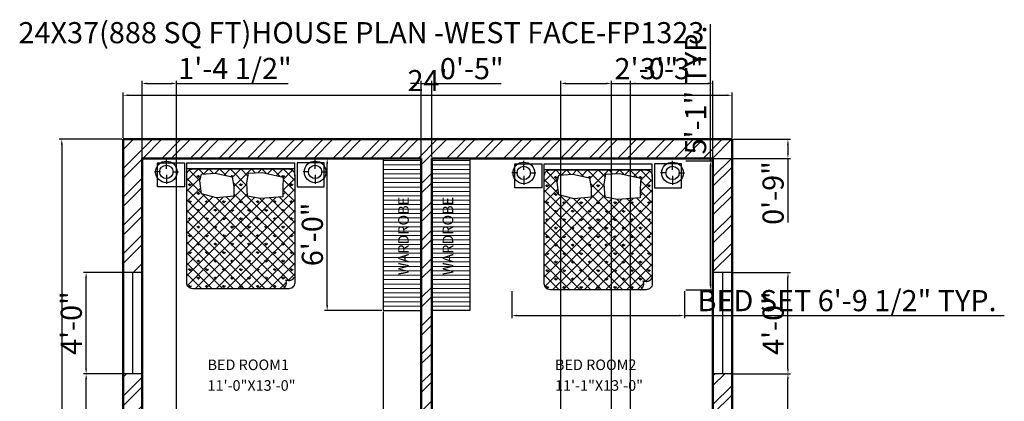
# Model space of a CAD drawing. Units: inches. Extents: x 3824 to 4289, y 1731 to 2259.
# Tile 5 of 5: x 3824 to 4289, y 2079 to 2259. Entities that reach past the tile are written whole.
import ezdxf

# ---------------------------------------------------------------- set-up
doc = ezdxf.new("R2010")
doc.units = ezdxf.units.IN
for name, color, linetype, lineweight in [('A-ANNO-DIMS', 2, 'Continuous', 18), ('A-ANNO-TEXT', 2, 'Continuous', 18), ('A-ANNO-TITL', 2, 'Continuous', 25), ('A-AREA-IDEN', 2, 'Continuous', 18), ('A-FLOR-CASE', 8, 'Continuous', 25), ('A-FURN', 9, 'Continuous', 18), ('WALL', 20, 'Continuous', 50), ('WINDOW', 4, 'Continuous', 25)]:
    doc.layers.add(name, color=color, linetype=linetype, lineweight=lineweight)
doc.layers.add('A-FLOR-CASE-PATT', color=251, linetype='Continuous', lineweight=13, true_color=0x636466)
doc.layers.add('A-WALL-PATT', color=251, linetype='Continuous', lineweight=13, true_color=0x636466)
doc.layers.add('GIUONG', color=70, linetype='Continuous')
doc.layers.add('NOI THAT', color=42, linetype='Continuous')
doc.styles.get("Standard").update_dxf_attribs({"font": 'arial.ttf'})
doc.dimstyles.new('ISO-25', dxfattribs={"dimtxt": 10, "dimasz": 2.5, "dimexe": 1.25, "dimexo": 0.625, "dimtad": 1, "dimdec": 1, "dimlunit": 3, "dimtxsty": 'Standard', "dimcen": 2.5, "dimadec": 0, "dimazin": 0, "dimtfac": 1, "dimtdec": 1, "dimtmove": 0, "dimatfit": 3, "dimfxl": 1, "dimarcsym": 0})

# ---------------------------------------------------------------- blocks, each defined once
blk = doc.blocks.new('*X4')
at = {"color": 0}
for p, q in [((0, 0), (0, 0)), ((-707, -141), (-734, -115)), ((-707, -141), (-707, -104)), ((-707, -141), (-681, -115)), ((-566, 0), (-566, 0)), ((-566, 0), (-566, 0)), ((-283, 0), (-283, 0)), ((-283, 0), (-283, 0)), ((-156, -126), (-168, -115)), ((-141, -141), (-142, -140)), ((-141, -141), (-141, -104)), ((-141, -141), (-115, -115)), ((120, -120), (115, -115)), ((283, 0), (283, 0)), ((566, 0), (566, 0)), ((699, -134), (681, -115)), ((707, -135), (707, -104)), ((710, -139), (734, -115)), ((-849, -283), (-875, -256)), ((-849, -283), (-849, -245)), ((-849, -283), (-822, -256)), ((0, -283), (-27, -256)), ((0, -283), (0, -245)), ((0, -283), (27, -256)), ((849, -283), (822, -256)), ((849, -283), (849, -245)), ((849, -283), (875, -256)), ((-707, -424), (-734, -398)), ((-707, -424), (-707, -387)), ((-707, -424), (-681, -398)), ((-116, -399), (-115, -398)), ((707, -424), (703, -420)), ((707, -424), (707, -387)), ((707, -424), (734, -398)), ((-849, -566), (-875, -539)), ((-849, -566), (-849, -528)), ((-849, -566), (-822, -539)), ((-566, -566), (-592, -539)), ((-566, -566), (-566, -528)), ((-566, -566), (-539, -539)), ((-283, -566), (-309, -539)), ((-283, -566), (-283, -528)), ((-283, -566), (-256, -539)), ((0, -566), (-27, -539)), ((0, -566), (0, -528)), ((0, -566), (27, -539)), ((283, -566), (256, -539)), ((283, -566), (283, -528)), ((283, -566), (309, -539)), ((566, -566), (539, -539)), ((566, -566), (566, -528)), ((566, -566), (592, -539)), ((849, -566), (822, -539)), ((849, -566), (849, -528)), ((849, -566), (875, -539)), ((-849, -849), (-849, -811)), ((-707, -707), (-734, -681)), ((-707, -707), (-707, -670)), ((-707, -707), (-681, -681)), ((-566, -849), (-566, -811)), ((-424, -707), (-451, -681)), ((-424, -707), (-424, -670)), ((-424, -707), (-398, -681)), ((-283, -849), (-283, -811)), ((-141, -707), (-168, -681)), ((-141, -707), (-141, -670)), ((-141, -707), (-115, -681)), ((0, -849), (0, -811)), ((141, -707), (115, -681)), ((141, -707), (141, -670)), ((141, -707), (168, -681)), ((283, -849), (283, -811)), ((424, -707), (398, -681)), ((424, -707), (424, -670)), ((424, -707), (451, -681)), ((566, -849), (566, -811)), ((707, -707), (681, -681)), ((707, -707), (707, -670)), ((707, -707), (734, -681)), ((849, -849), (849, -811)), ((-849, -849), (-875, -822)), ((-849, -849), (-822, -822)), ((-707, -990), (-734, -963)), ((-707, -990), (-707, -952)), ((-707, -990), (-681, -963)), ((-566, -849), (-592, -822)), ((-566, -849), (-539, -822)), ((-424, -990), (-451, -963)), ((-424, -990), (-424, -952)), ((-424, -990), (-398, -963)), ((-283, -849), (-309, -822)), ((-283, -849), (-256, -822)), ((-141, -990), (-168, -963)), ((-141, -990), (-141, -952)), ((-141, -990), (-115, -963)), ((0, -849), (-27, -822)), ((0, -849), (27, -822)), ((141, -990), (115, -963)), ((141, -990), (141, -952)), ((141, -990), (168, -963)), ((283, -849), (256, -822)), ((283, -849), (309, -822)), ((424, -990), (398, -963)), ((424, -990), (424, -952)), ((424, -990), (451, -963)), ((566, -849), (539, -822)), ((566, -849), (592, -822)), ((707, -990), (681, -963)), ((707, -990), (707, -952)), ((707, -990), (734, -963)), ((849, -849), (822, -822)), ((849, -849), (875, -822)), ((-849, -1131), (-875, -1105)), ((-849, -1131), (-849, -1094)), ((-849, -1131), (-822, -1105)), ((-566, -1131), (-592, -1105)), ((-566, -1131), (-566, -1094)), ((-566, -1131), (-539, -1105)), ((-283, -1131), (-309, -1105)), ((-283, -1131), (-283, -1094)), ((-283, -1131), (-256, -1105)), ((0, -1131), (-27, -1105)), ((0, -1131), (0, -1094)), ((0, -1131), (27, -1105)), ((283, -1131), (256, -1105)), ((283, -1131), (283, -1094)), ((283, -1131), (309, -1105)), ((566, -1131), (539, -1105)), ((566, -1131), (566, -1094)), ((566, -1131), (592, -1105)), ((849, -1131), (822, -1105)), ((849, -1131), (849, -1094)), ((849, -1131), (875, -1105)), ((-707, -1273), (-734, -1246)), ((-707, -1273), (-707, -1235)), ((-707, -1273), (-681, -1246)), ((-424, -1273), (-451, -1246)), ((-424, -1273), (-424, -1235)), ((-424, -1273), (-398, -1246)), ((-141, -1273), (-168, -1246)), ((-141, -1273), (-141, -1235)), ((-141, -1273), (-115, -1246)), ((141, -1273), (115, -1246)), ((141, -1273), (141, -1235)), ((141, -1273), (168, -1246)), ((424, -1273), (398, -1246)), ((424, -1273), (424, -1235)), ((424, -1273), (451, -1246)), ((707, -1273), (681, -1246)), ((707, -1273), (707, -1235)), ((707, -1273), (734, -1246)), ((-849, -1414), (-875, -1388)), ((-849, -1414), (-849, -1377)), ((-849, -1414), (-822, -1388)), ((-566, -1414), (-592, -1388)), ((-566, -1414), (-566, -1377)), ((-566, -1414), (-539, -1388)), ((-283, -1414), (-309, -1388)), ((-283, -1414), (-283, -1377)), ((-283, -1414), (-256, -1388)), ((0, -1414), (-27, -1388)), ((0, -1414), (0, -1377)), ((0, -1414), (27, -1388)), ((283, -1414), (256, -1388)), ((283, -1414), (283, -1377)), ((283, -1414), (309, -1388)), ((566, -1414), (539, -1388)), ((566, -1414), (566, -1377)), ((566, -1414), (592, -1388)), ((849, -1414), (822, -1388)), ((849, -1414), (849, -1377)), ((849, -1414), (875, -1388)), ((-707, -1556), (-734, -1529)), ((-707, -1556), (-707, -1518)), ((-707, -1556), (-681, -1529)), ((-424, -1556), (-451, -1529)), ((-424, -1556), (-424, -1518)), ((-424, -1556), (-398, -1529)), ((-141, -1556), (-168, -1529)), ((-141, -1556), (-141, -1518)), ((-141, -1556), (-115, -1529)), ((141, -1556), (115, -1529)), ((141, -1556), (141, -1518)), ((141, -1556), (168, -1529)), ((424, -1556), (398, -1529)), ((424, -1556), (424, -1518)), ((424, -1556), (451, -1529)), ((707, -1556), (681, -1529)), ((707, -1556), (707, -1518)), ((707, -1556), (734, -1529)), ((-849, -1697), (-875, -1671)), ((-849, -1697), (-849, -1660)), ((-849, -1697), (-822, -1671)), ((-707, -1838), (-707, -1801)), ((-566, -1697), (-592, -1671)), ((-566, -1697), (-566, -1660)), ((-566, -1697), (-539, -1671)), ((-424, -1838), (-424, -1801)), ((-283, -1697), (-309, -1671)), ((-283, -1697), (-283, -1660)), ((-283, -1697), (-256, -1671)), ((-141, -1838), (-141, -1801)), ((0, -1697), (-27, -1671)), ((0, -1697), (0, -1660)), ((0, -1697), (27, -1671)), ((141, -1838), (141, -1801)), ((283, -1697), (256, -1671)), ((283, -1697), (283, -1660)), ((283, -1697), (309, -1671)), ((424, -1838), (424, -1801)), ((566, -1697), (539, -1671)), ((566, -1697), (566, -1660)), ((566, -1697), (592, -1671)), ((707, -1838), (707, -1801)), ((849, -1697), (822, -1671)), ((849, -1697), (849, -1660)), ((849, -1697), (875, -1671)), ((-849, -1980), (-875, -1953)), ((-849, -1980), (-849, -1942)), ((-849, -1980), (-822, -1953)), ((-707, -1838), (-734, -1812)), ((-707, -1838), (-681, -1812)), ((-566, -1980), (-592, -1953)), ((-566, -1980), (-566, -1942)), ((-566, -1980), (-539, -1953)), ((-424, -1838), (-451, -1812)), ((-424, -1838), (-398, -1812)), ((-283, -1980), (-309, -1953)), ((-283, -1980), (-283, -1942)), ((-283, -1980), (-256, -1953)), ((-141, -1838), (-168, -1812)), ((-141, -1838), (-115, -1812)), ((0, -1980), (-27, -1953)), ((0, -1980), (0, -1942)), ((0, -1980), (27, -1953)), ((141, -1838), (115, -1812)), ((141, -1838), (168, -1812)), ((283, -1980), (256, -1953)), ((283, -1980), (283, -1942)), ((283, -1980), (309, -1953)), ((424, -1838), (398, -1812)), ((424, -1838), (451, -1812)), ((566, -1980), (539, -1953)), ((566, -1980), (566, -1942)), ((566, -1980), (592, -1953)), ((707, -1838), (681, -1812)), ((707, -1838), (734, -1812))]:
    blk.add_line(p, q, dxfattribs=at)
blk = doc.blocks.new('*X3')
at = {"color": 0}
for p, q in [((-900, -193), (-707, 0)), ((-623, -84), (-707, 0)), ((-614, -83), (-530, 0)), ((-457, -74), (-530, 0)), ((-425, -72), (-354, 0)), ((-245, -108), (-354, 0)), ((-278, -101), (-177, 0)), ((103, -280), (-177, 0)), ((-142, -142), (0, 0)), ((-117, -294), (177, 0)), ((120, -120), (0, 0)), ((241, -64), (177, 0)), ((292, -61), (354, 0)), ((426, -72), (354, 0)), ((452, -78), (530, 0)), ((654, -123), (530, 0)), ((596, -111), (707, 0)), ((900, -193), (707, 0)), ((-900, -370), (-667, -137)), ((-656, -405), (-900, -161)), ((-683, -201), (-862, -22)), ((703, -358), (900, -161)), ((708, -175), (862, -22)), ((-900, -1254), (101, -252)), ((-900, -546), (-668, -314)), ((900, -1254), (-128, -225)), ((900, -370), (708, -178)), ((735, -1973), (-900, -337)), ((-900, -1430), (112, -418)), ((-900, -723), (-605, -429)), ((-900, -900), (-465, -465)), ((-900, -1077), (-293, -470)), ((-900, -1607), (231, -476)), ((-900, -1784), (394, -489)), ((-888, -1948), (586, -475)), ((-763, -2000), (900, -337)), ((801, -1862), (-641, -419)), ((900, -1784), (-404, -480)), ((900, -1607), (-243, -465)), ((900, -1430), (-116, -415)), ((900, -900), (483, -483)), ((900, -723), (647, -470)), ((900, -546), (703, -349)), ((586, -2000), (-900, -514)), ((-586, -2000), (900, -514)), ((900, -1077), (317, -494)), ((409, -2000), (-900, -691)), ((-409, -2000), (900, -691)), ((232, -2000), (-900, -868)), ((-232, -2000), (900, -868)), ((55, -2000), (-900, -1045)), ((-55, -2000), (900, -1045)), ((-121, -2000), (-900, -1221)), ((121, -2000), (900, -1221)), ((-298, -2000), (-900, -1398)), ((298, -2000), (900, -1398)), ((-475, -2000), (-900, -1575)), ((475, -2000), (900, -1575)), ((-652, -2000), (-900, -1752)), ((790, -1861), (900, -1752)), ((-835, -1994), (-894, -1935)), ((652, -2000), (761, -1890))]:
    blk.add_line(p, q, dxfattribs=at)
blk = doc.blocks.new('A$C190D2546')
at = {"layer": 'GIUONG'}
for points in [[(787, 1584), (758, 1799), (787, 1914), (1016, 1928), (1296, 1871), (1325, 1699), (1325, 1548), (1038, 1519)], [(1555, 1548), (1541, 1771), (1569, 1928), (1799, 1943), (2151, 1864), (2144, 1685), (2144, 1534), (1763, 1505)]]:
    blk.add_lwpolyline(points, close=True, dxfattribs=at)
for centre, radius in [((200, 1951), 180), ((200, 1951), 112), ((2682, 1951), 180), ((2682, 1951), 112)]:
    blk.add_circle(centre, radius, dxfattribs=at)
at = {"layer": 'NOI THAT'}
for p, q in [((200, 2001), (200, 2151)), ((2682, 2001), (2682, 2151)), ((541, 2100), (2341, 2100)), ((541, 1881), (541, 2100)), ((2341, 2000), (541, 2000)), ((2341, 1881), (2341, 2100)), ((100, 1951), (0, 1951)), ((200, 1901), (200, 1751)), ((300, 1951), (400, 1951)), ((2582, 1951), (2482, 1951)), ((2682, 1901), (2682, 1751)), ((2782, 1951), (2882, 1951))]:
    blk.add_line(p, q, dxfattribs=at)
for points in [[(500, 2101), (500, 1701), (50, 1701), (50, 2101)], [(2382, 2101), (2382, 1701), (2832, 1701), (2832, 2101)]]:
    blk.add_lwpolyline(points, close=True, dxfattribs=at)
blk.add_lwpolyline([(641, 2000), (2241, 2000, -0.414214), (2341, 1900), (2341, 100, -0.414214), (2241, 0), (641, 0, -0.414214), (541, 100), (541, 1900, -0.414214)], format="xyb", close=True, dxfattribs=at)
for centre, start, end in [((2241, 250), 243.4349, 333.4349), ((2091, 100), 296.5651, 26.5651)]:
    blk.add_arc(centre, 112, start, end, dxfattribs=at)
for name in ['*X3', '*X4']:
    blk.add_blockref(name, (1441, 2000), dxfattribs=at)
blk = doc.blocks.new('*D11')
at = {"layer": 'A-ANNO-DIMS', "color": 0, "lineweight": -2, "transparency": 16777216}
for p, q in [((3872.55, 2203.24), (3872.55, 2224.73)), ((3875.05, 2223.48), (4158.05, 2223.48)), ((4160.55, 2203.24), (4160.55, 2224.73))]:
    blk.add_line(p, q, dxfattribs=at)
at = {"layer": 'A-ANNO-DIMS', "color": 0, "transparency": 16777216}
for points in [[(3875.05, 2223.9), (3875.05, 2223.07), (3872.55, 2223.48)], [(4158.05, 2223.9), (4158.05, 2223.07), (4160.55, 2223.48)]]:
    blk.add_solid(points, dxfattribs=at)
at = {"layer": 'Defpoints', "color": 0, "transparency": 16777216}
for p in [(4160.55, 2223.48), (3872.55, 2202.62), (4160.55, 2202.62)]:
    blk.add_point(p, dxfattribs=at)
at = {"layer": 'A-ANNO-DIMS', "color": 0, "transparency": 16777216, "insert": (4016.55, 2229.13), "char_height": 10, "attachment_point": 5}
blk.add_mtext("24'", dxfattribs=at)
blk = doc.blocks.new('*D12')
at = {"layer": 'A-ANNO-DIMS', "color": 0, "lineweight": -2, "transparency": 16777216}
for p, q in [((3871.93, 2202.62), (3842.32, 2202.62)), ((3843.57, 2200.12), (3843.57, 1761.12)), ((3871.93, 1758.62), (3842.32, 1758.62))]:
    blk.add_line(p, q, dxfattribs=at)
at = {"layer": 'A-ANNO-DIMS', "color": 0, "transparency": 16777216}
for points in [[(3843.15, 2200.12), (3843.99, 2200.12), (3843.57, 2202.62)], [(3843.15, 1761.12), (3843.99, 1761.12), (3843.57, 1758.62)]]:
    blk.add_solid(points, dxfattribs=at)
at = {"layer": 'Defpoints', "color": 0, "transparency": 16777216}
for p in [(3872.55, 2202.62), (3843.57, 1758.62), (3872.55, 1758.62)]:
    blk.add_point(p, dxfattribs=at)
at = {"layer": 'A-ANNO-DIMS', "color": 0, "transparency": 16777216, "insert": (3837.84, 1980.62), "char_height": 10, "attachment_point": 5, "rotation": 90}
blk.add_mtext("37'", dxfattribs=at)
blk = doc.blocks.new('*D14')
at = {"layer": 'A-ANNO-DIMS', "color": 0, "lineweight": -2, "transparency": 16777216}
for p, q in [((4056.41, 2130.79), (4056.41, 2117.92)), ((4138.1, 2130.79), (4138.1, 2117.92)), ((4058.91, 2119.17), (4135.6, 2119.17)), ((4138.1, 2119.17), (4289.32, 2119.17))]:
    blk.add_line(p, q, dxfattribs=at)
at = {"layer": 'A-ANNO-DIMS', "color": 0, "transparency": 16777216}
for points in [[(4058.91, 2119.58), (4058.91, 2118.75), (4056.41, 2119.17)], [(4135.6, 2119.58), (4135.6, 2118.75), (4138.1, 2119.17)]]:
    blk.add_solid(points, dxfattribs=at)
at = {"layer": 'Defpoints', "color": 0, "transparency": 16777216}
for p in [(4056.41, 2131.42), (4138.1, 2131.42), (4138.1, 2119.17)]:
    blk.add_point(p, dxfattribs=at)
at = {"layer": 'A-ANNO-DIMS', "color": 0, "transparency": 16777216, "insert": (4214.96, 2124.96), "char_height": 10, "attachment_point": 5}
blk.add_mtext('BED SET 6\'-9 1/2" TYP.', dxfattribs=at)
blk = doc.blocks.new('*D15')
at = {"layer": 'A-ANNO-DIMS', "color": 0, "lineweight": -2, "transparency": 16777216}
for p, q in [((4150.35, 2192.38), (4150.35, 2257.09)), ((4138.72, 2192.38), (4151.6, 2192.38)), ((4150.35, 2133.92), (4150.35, 2189.88)), ((4138.72, 2131.42), (4151.6, 2131.42))]:
    blk.add_line(p, q, dxfattribs=at)
at = {"layer": 'A-ANNO-DIMS', "color": 0, "transparency": 16777216}
for points in [[(4149.93, 2189.88), (4150.77, 2189.88), (4150.35, 2192.38)], [(4149.93, 2133.92), (4150.77, 2133.92), (4150.35, 2131.42)]]:
    blk.add_solid(points, dxfattribs=at)
at = {"layer": 'Defpoints', "color": 0, "transparency": 16777216}
for p in [(4138.1, 2192.38), (4150.35, 2192.38), (4138.1, 2131.42)]:
    blk.add_point(p, dxfattribs=at)
at = {"layer": 'A-ANNO-DIMS', "color": 0, "transparency": 16777216, "insert": (4144.62, 2225.98), "char_height": 10, "attachment_point": 5, "rotation": 90}
blk.add_mtext('5\'-1" TYP.', dxfattribs=at)
blk = doc.blocks.new('*D30')
at = {"layer": 'A-ANNO-DIMS', "color": 0, "lineweight": -2, "transparency": 16777216}
for p, q in [((3880.93, 2091.62), (3853.85, 2091.62)), ((3855.1, 2017.12), (3855.1, 2089.12)), ((3880.93, 2014.62), (3853.85, 2014.62))]:
    blk.add_line(p, q, dxfattribs=at)
at = {"layer": 'A-ANNO-DIMS', "color": 0, "transparency": 16777216}
for points in [[(3854.69, 2089.12), (3855.52, 2089.12), (3855.1, 2091.62)], [(3854.69, 2017.12), (3855.52, 2017.12), (3855.1, 2014.62)]]:
    blk.add_solid(points, dxfattribs=at)
at = {"layer": 'Defpoints', "color": 0, "transparency": 16777216}
for p in [(3855.1, 2091.62), (3881.55, 2091.62), (3881.55, 2014.62)]:
    blk.add_point(p, dxfattribs=at)
at = {"layer": 'A-ANNO-DIMS', "color": 0, "transparency": 16777216, "insert": (3849.37, 2053.12), "char_height": 10, "attachment_point": 5, "rotation": 90}
blk.add_mtext('6\'-5"', dxfattribs=at)
blk = doc.blocks.new('*D31')
at = {"layer": 'A-ANNO-DIMS', "color": 0, "lineweight": -2, "transparency": 16777216}
for p, q in [((3880.93, 2139.62), (3853.85, 2139.62)), ((3855.1, 2094.12), (3855.1, 2137.12)), ((3880.93, 2091.62), (3853.85, 2091.62))]:
    blk.add_line(p, q, dxfattribs=at)
at = {"layer": 'A-ANNO-DIMS', "color": 0, "transparency": 16777216}
for points in [[(3854.69, 2137.12), (3855.52, 2137.12), (3855.1, 2139.62)], [(3854.69, 2094.12), (3855.52, 2094.12), (3855.1, 2091.62)]]:
    blk.add_solid(points, dxfattribs=at)
at = {"layer": 'Defpoints', "color": 0, "transparency": 16777216}
for p in [(3855.1, 2139.62), (3881.55, 2139.62), (3881.55, 2091.62)]:
    blk.add_point(p, dxfattribs=at)
at = {"layer": 'A-ANNO-DIMS', "color": 0, "transparency": 16777216, "insert": (3849.37, 2115.62), "char_height": 10, "attachment_point": 5, "rotation": 90}
blk.add_mtext('4\'-0"', dxfattribs=at)
blk = doc.blocks.new('*D36')
at = {"layer": 'A-ANNO-DIMS', "color": 0, "lineweight": -2, "transparency": 16777216}
for p, q in [((4161.18, 2091.62), (4188.25, 2091.62)), ((4187, 2011.12), (4187, 2089.12)), ((4161.18, 2008.62), (4188.25, 2008.62))]:
    blk.add_line(p, q, dxfattribs=at)
at = {"layer": 'A-ANNO-DIMS', "color": 0, "transparency": 16777216}
for points in [[(4186.59, 2089.12), (4187.42, 2089.12), (4187, 2091.62)], [(4186.59, 2011.12), (4187.42, 2011.12), (4187, 2008.62)]]:
    blk.add_solid(points, dxfattribs=at)
at = {"layer": 'Defpoints', "color": 0, "transparency": 16777216}
for p in [(4160.55, 2091.62), (4187, 2091.62), (4160.55, 2008.62)]:
    blk.add_point(p, dxfattribs=at)
at = {"layer": 'A-ANNO-DIMS', "color": 0, "transparency": 16777216, "insert": (4181.27, 2050.12), "char_height": 10, "attachment_point": 5, "rotation": 90}
blk.add_mtext('6\'-11"', dxfattribs=at)
blk = doc.blocks.new('*D37')
at = {"layer": 'A-ANNO-DIMS', "color": 0, "lineweight": -2, "transparency": 16777216}
for p, q in [((4161.18, 2139.62), (4188.25, 2139.62)), ((4187, 2094.12), (4187, 2137.12)), ((4161.18, 2091.62), (4188.25, 2091.62))]:
    blk.add_line(p, q, dxfattribs=at)
at = {"layer": 'A-ANNO-DIMS', "color": 0, "transparency": 16777216}
for points in [[(4186.59, 2137.12), (4187.42, 2137.12), (4187, 2139.62)], [(4186.59, 2094.12), (4187.42, 2094.12), (4187, 2091.62)]]:
    blk.add_solid(points, dxfattribs=at)
at = {"layer": 'Defpoints', "color": 0, "transparency": 16777216}
for p in [(4160.55, 2139.62), (4187, 2139.62), (4160.55, 2091.62)]:
    blk.add_point(p, dxfattribs=at)
at = {"layer": 'A-ANNO-DIMS', "color": 0, "transparency": 16777216, "insert": (4181.27, 2115.62), "char_height": 10, "attachment_point": 5, "rotation": 90}
blk.add_mtext('4\'-0"', dxfattribs=at)
blk = doc.blocks.new('*D50')
at = {"layer": 'A-ANNO-DIMS', "color": 0, "lineweight": -2, "transparency": 16777216}
for p, q in [((4079.55, 1818.24), (4079.55, 2230.32)), ((4082.05, 2229.07), (4101.05, 2229.07)), ((4103.55, 1818.24), (4103.55, 2230.32)), ((4103.55, 2229.07), (4134.06, 2229.07))]:
    blk.add_line(p, q, dxfattribs=at)
at = {"layer": 'A-ANNO-DIMS', "color": 0, "transparency": 16777216}
for points in [[(4082.05, 2229.49), (4082.05, 2228.65), (4079.55, 2229.07)], [(4101.05, 2229.49), (4101.05, 2228.65), (4103.55, 2229.07)]]:
    blk.add_solid(points, dxfattribs=at)
at = {"layer": 'Defpoints', "color": 0, "transparency": 16777216}
for p in [(4103.55, 2229.07), (4079.55, 1817.62), (4103.55, 1817.62)]:
    blk.add_point(p, dxfattribs=at)
at = {"layer": 'A-ANNO-DIMS', "color": 0, "transparency": 16777216, "insert": (4120.05, 2234.8), "char_height": 10, "attachment_point": 5}
blk.add_mtext('2\'-0"', dxfattribs=at)
blk = doc.blocks.new('*D51')
at = {"layer": 'A-ANNO-DIMS', "color": 0, "lineweight": -2, "transparency": 16777216}
for p, q in [((4112.55, 1917.24), (4112.55, 2230.32)), ((4115.05, 2229.07), (4149.05, 2229.07)), ((4151.55, 1917.24), (4151.55, 2230.32))]:
    blk.add_line(p, q, dxfattribs=at)
at = {"layer": 'A-ANNO-DIMS', "color": 0, "transparency": 16777216}
for points in [[(4115.05, 2229.49), (4115.05, 2228.65), (4112.55, 2229.07)], [(4149.05, 2229.49), (4149.05, 2228.65), (4151.55, 2229.07)]]:
    blk.add_solid(points, dxfattribs=at)
at = {"layer": 'Defpoints', "color": 0, "transparency": 16777216}
for p in [(4151.55, 2229.07), (4112.55, 1916.62), (4151.55, 1916.62)]:
    blk.add_point(p, dxfattribs=at)
at = {"layer": 'A-ANNO-DIMS', "color": 0, "transparency": 16777216, "insert": (4132.05, 2234.8), "char_height": 10, "attachment_point": 5}
blk.add_mtext('3\'-3"', dxfattribs=at)
blk = doc.blocks.new('*D54')
at = {"layer": 'A-ANNO-DIMS', "color": 0, "lineweight": -2, "transparency": 16777216}
for p, q in [((4161.18, 2202.62), (4188.25, 2202.62)), ((4187, 2200.12), (4187, 2196.12)), ((4152.18, 2193.62), (4188.25, 2193.62)), ((4187, 2193.62), (4187, 2163.29))]:
    blk.add_line(p, q, dxfattribs=at)
at = {"layer": 'A-ANNO-DIMS', "color": 0, "transparency": 16777216}
for points in [[(4186.59, 2200.12), (4187.42, 2200.12), (4187, 2202.62)], [(4186.59, 2196.12), (4187.42, 2196.12), (4187, 2193.62)]]:
    blk.add_solid(points, dxfattribs=at)
at = {"layer": 'Defpoints', "color": 0, "transparency": 16777216}
for p in [(4160.55, 2202.62), (4151.55, 2193.62), (4187, 2193.62)]:
    blk.add_point(p, dxfattribs=at)
at = {"layer": 'A-ANNO-DIMS', "color": 0, "transparency": 16777216, "insert": (4181.27, 2177.2), "char_height": 10, "attachment_point": 5, "rotation": 90}
blk.add_mtext('0\'-9"', dxfattribs=at)
blk = doc.blocks.new('*D55')
at = {"layer": 'A-ANNO-DIMS', "color": 0, "lineweight": -2, "transparency": 16777216}
for p, q in [((4011.05, 2229.07), (4008.55, 2229.07)), ((4013.55, 2194.24), (4013.55, 2230.32)), ((4013.55, 2229.07), (4018.55, 2229.07)), ((4018.55, 2194.24), (4018.55, 2230.32)), ((4021.05, 2229.07), (4051.38, 2229.07))]:
    blk.add_line(p, q, dxfattribs=at)
at = {"layer": 'A-ANNO-DIMS', "color": 0, "transparency": 16777216}
for points in [[(4011.05, 2229.49), (4011.05, 2228.65), (4013.55, 2229.07)], [(4021.05, 2229.49), (4021.05, 2228.65), (4018.55, 2229.07)]]:
    blk.add_solid(points, dxfattribs=at)
at = {"layer": 'Defpoints', "color": 0, "transparency": 16777216}
for p in [(4018.55, 2229.07), (4013.55, 2193.62), (4018.55, 2193.62)]:
    blk.add_point(p, dxfattribs=at)
at = {"layer": 'A-ANNO-DIMS', "color": 0, "transparency": 16777216, "insert": (4037.47, 2234.8), "char_height": 10, "attachment_point": 5}
blk.add_mtext('0\'-5"', dxfattribs=at)
blk = doc.blocks.new('*D56')
at = {"layer": 'A-ANNO-DIMS', "color": 0, "lineweight": -2, "transparency": 16777216}
for p, q in [((3995.55, 2120.99), (3995.55, 1730.92)), ((4013.55, 2120.99), (4013.55, 1730.92)), ((3998.05, 1732.17), (4011.05, 1732.17)), ((4013.55, 1732.17), (4042.94, 1732.17))]:
    blk.add_line(p, q, dxfattribs=at)
at = {"layer": 'A-ANNO-DIMS', "color": 0, "transparency": 16777216}
for points in [[(3998.05, 1732.59), (3998.05, 1731.75), (3995.55, 1732.17)], [(4011.05, 1732.59), (4011.05, 1731.75), (4013.55, 1732.17)]]:
    blk.add_solid(points, dxfattribs=at)
at = {"layer": 'Defpoints', "color": 0, "transparency": 16777216}
for p in [(3995.55, 2121.62), (4013.55, 2121.62), (4013.55, 1732.17)]:
    blk.add_point(p, dxfattribs=at)
at = {"layer": 'A-ANNO-DIMS', "color": 0, "transparency": 16777216, "insert": (4029.5, 1737.9), "char_height": 10, "attachment_point": 5}
blk.add_mtext('1\'-6"', dxfattribs=at)
blk = doc.blocks.new('*D57')
at = {"layer": 'A-ANNO-DIMS', "color": 0, "lineweight": -2, "transparency": 16777216}
for p, q in [((3994.93, 2193.62), (3967.85, 2193.62)), ((3969.1, 2124.12), (3969.1, 2191.12)), ((3994.93, 2121.62), (3967.85, 2121.62))]:
    blk.add_line(p, q, dxfattribs=at)
at = {"layer": 'A-ANNO-DIMS', "color": 0, "transparency": 16777216}
for points in [[(3968.69, 2191.12), (3969.52, 2191.12), (3969.1, 2193.62)], [(3968.69, 2124.12), (3969.52, 2124.12), (3969.1, 2121.62)]]:
    blk.add_solid(points, dxfattribs=at)
at = {"layer": 'Defpoints', "color": 0, "transparency": 16777216}
for p in [(3969.1, 2193.62), (3995.55, 2193.62), (3995.55, 2121.62)]:
    blk.add_point(p, dxfattribs=at)
at = {"layer": 'A-ANNO-DIMS', "color": 0, "transparency": 16777216, "insert": (3963.37, 2157.62), "char_height": 10, "attachment_point": 5, "rotation": 90}
blk.add_mtext('6\'-0"', dxfattribs=at)
blk = doc.blocks.new('*D59')
at = {"layer": 'A-ANNO-DIMS', "color": 0, "lineweight": -2, "transparency": 16777216}
for p, q in [((3881.55, 2033.24), (3881.55, 2230.32)), ((3884.05, 2229.07), (3895.39, 2229.07)), ((3897.89, 2033.24), (3897.89, 2230.32)), ((3897.89, 2229.07), (3950.58, 2229.07))]:
    blk.add_line(p, q, dxfattribs=at)
at = {"layer": 'A-ANNO-DIMS', "color": 0, "transparency": 16777216}
for points in [[(3884.05, 2229.49), (3884.05, 2228.65), (3881.55, 2229.07)], [(3895.39, 2229.49), (3895.39, 2228.65), (3897.89, 2229.07)]]:
    blk.add_solid(points, dxfattribs=at)
at = {"layer": 'Defpoints', "color": 0, "transparency": 16777216}
for p in [(3897.89, 2229.07), (3881.55, 2032.62), (3897.89, 2032.62)]:
    blk.add_point(p, dxfattribs=at)
at = {"layer": 'A-ANNO-DIMS', "color": 0, "transparency": 16777216, "insert": (3925.49, 2234.86), "char_height": 10, "attachment_point": 5}
blk.add_mtext('1\'-4 1/2"', dxfattribs=at)

msp = doc.modelspace()

# ---------------------------------------------------------------- hatches: boundary and pattern name
at = {"layer": 'A-FLOR-CASE-PATT'}
h = msp.add_hatch(dxfattribs=at)
h.set_pattern_fill('ANSI31', color=256, scale=0.65769, angle=-45, style=0)
h.paths.add_polyline_path([(3995.55, 2121.62), (4013.55, 2121.62), (4013.55, 2193.62), (3995.55, 2193.62)])
h = msp.add_hatch(dxfattribs=at)
h.set_pattern_fill('ANSI31', color=256, scale=0.65769, angle=-45, style=0)
h.paths.add_polyline_path([(4018.55, 2121.62), (4036.55, 2121.62), (4036.55, 2193.62), (4018.55, 2193.62)])
at = {"layer": 'A-WALL-PATT'}
h = msp.add_hatch(dxfattribs=at)
h.set_pattern_fill('ANSI32', color=256)
h.paths.add_polyline_path([(4160.55, 2202.62), (3872.55, 2202.62), (3872.55, 2139.62), (3881.55, 2139.62), (3881.55, 2193.62), (4013.55, 2193.62), (4013.55, 2037.62), (4004.55, 2037.62), (4004.55, 2032.62), (4027.55, 2032.62), (4027.55, 2037.62), (4018.55, 2037.62), (4018.55, 2193.62), (4036.55, 2193.62), (4151.55, 2193.62), (4151.55, 2139.62), (4160.55, 2139.62)])
h = msp.add_hatch(dxfattribs=at)
h.set_pattern_fill('ANSI32', color=256)
h.paths.add_polyline_path([(3881.55, 2091.62), (3872.55, 2091.62), (3872.55, 2014.62), (3881.55, 2014.62), (3881.55, 2032.62), (3897.89, 2032.62), (3968.55, 2032.62), (3968.55, 2037.62), (3881.55, 2037.62)])
h = msp.add_hatch(dxfattribs=at)
h.set_pattern_fill('ANSI32', color=256)
h.paths.add_polyline_path([(4160.55, 2091.62), (4151.55, 2091.62), (4151.55, 2037.62), (4063.55, 2037.62), (4063.55, 2032.62), (4151.55, 2032.62), (4151.55, 2008.62), (4160.55, 2008.62)])

# ---------------------------------------------------------------- linework, layer by layer
at = {"layer": 'A-FLOR-CASE'}
for p, q in [((4013.55, 2193.62), (3995.55, 2193.62)), ((3995.55, 2193.62), (3995.55, 2121.62)), ((4018.55, 2193.62), (4036.55, 2193.62)), ((4036.55, 2193.62), (4036.55, 2121.62)), ((3995.55, 2121.62), (4013.55, 2121.62)), ((4036.55, 2121.62), (4018.55, 2121.62))]:
    msp.add_line(p, q, dxfattribs=at)
at = {"layer": 'WALL'}
for p, q in [((3872.55, 2202.62), (4160.55, 2202.62)), ((3872.55, 2202.62), (3872.55, 1758.62)), ((4160.55, 2202.62), (4160.55, 1758.62)), ((3881.55, 2193.62), (4013.55, 2193.62)), ((3881.55, 2193.62), (3881.55, 2037.62)), ((4013.55, 2193.62), (4013.55, 2037.62)), ((4018.55, 2193.62), (4018.55, 2037.62)), ((4018.55, 2193.62), (4151.55, 2193.62)), ((4151.55, 2193.62), (4151.55, 2037.62))]:
    msp.add_line(p, q, dxfattribs=at)
at = {"layer": 'WINDOW'}
for p, q in [((3881.55, 2139.62), (3872.55, 2139.62)), ((3877.05, 2139.62), (3877.05, 2091.62)), ((4160.55, 2139.62), (4151.55, 2139.62)), ((4156.05, 2139.62), (4156.05, 2091.62)), ((3881.55, 2091.62), (3872.55, 2091.62)), ((4160.55, 2091.62), (4151.55, 2091.62))]:
    msp.add_line(p, q, dxfattribs=at)

# ---------------------------------------------------------------- block references
at = {"layer": 'A-FURN', "xscale": 0.0283444227516291, "yscale": 0.0283444227516291, "zscale": 0.0283444227516291}
for p in [(3887.38, 2131.9), (4056.41, 2131.42)]:
    msp.add_blockref('A$C190D2546', p, dxfattribs=at)

# ---------------------------------------------------------------- texts
at = {"layer": 'A-ANNO-TEXT'}
for p in [(4007.67, 2138.32), (4028.7, 2138.32)]:
    msp.add_text('WARDROBE', height=5, rotation=90, dxfattribs=at).set_placement(p)
at = {"layer": 'A-ANNO-TITL'}
msp.add_text('24X37(888 SQ FT)HOUSE PLAN -WEST FACE-FP1323', height=10, dxfattribs=at).set_placement((3823.13, 2248.11))
at = {"layer": 'A-AREA-IDEN'}
for s, p in [('BED ROOM1', (3912.51, 2093.38)), ('BED ROOM2', (4076.84, 2093.38)), ('11\'-0"X13\'-0"', (3912.51, 2083.59)), ('11\'-1"X13\'-0"', (4076.84, 2083.59))]:
    msp.add_text(s, height=5, dxfattribs=at).set_placement(p)

# ---------------------------------------------------------------- dimensions: what is measured, and where the dimension line sits
at = {"layer": 'A-ANNO-DIMS'}
dim = msp.add_linear_dim(base=(4150.35, 2192.38), p1=(4138.1, 2131.42), p2=(4138.1, 2192.38), angle=90, text='<> TYP.', dimstyle='ISO-25', override={"dimdec": 1, "dimlfac": 1, "dimrnd": 0, "dimzin": 1, "dimdsep": 46, "dimlunit": 4, "dimfrac": 2}, dxfattribs=at)
dim.commit()
dim.dimension.update_dxf_attribs({"geometry": '*D15', "text_midpoint": (4144.62, 2225.98)})
for base, p1, p2, override, picture, middle in [((3897.89, 2229.07), (3881.55, 2032.62), (3897.89, 2032.62), {"dimdec": 1, "dimlfac": 1, "dimrnd": 0, "dimzin": 1, "dimdsep": 46, "dimlunit": 4, "dimfrac": 2}, '*D59', (3925.49, 2234.86)), ((4018.55, 2229.07), (4013.55, 2193.62), (4018.55, 2193.62), {"dimdec": 1, "dimlfac": 1, "dimrnd": 0, "dimzin": 1, "dimdsep": 46, "dimlunit": 4, "dimfrac": 2}, '*D55', (4037.47, 2234.8)), ((4103.55, 2229.07), (4079.55, 1817.62), (4103.55, 1817.62), {"dimdec": 1, "dimlfac": 1, "dimrnd": 0, "dimzin": 1, "dimdsep": 46, "dimlunit": 4, "dimfrac": 2}, '*D50', (4120.05, 2234.8)), ((4151.55, 2229.07), (4112.55, 1916.62), (4151.55, 1916.62), {"dimdec": 1, "dimlfac": 1, "dimrnd": 0, "dimzin": 1, "dimdsep": 46, "dimlunit": 4, "dimfrac": 2}, '*D51', (4132.05, 2234.8)), ((4160.55, 2223.48), (3872.55, 2202.62), (4160.55, 2202.62), {"dimclrd": 0, "dimclre": 0, "dimclrt": 0}, '*D11', (4016.55, 2229.13)), ((4013.55, 1732.17), (3995.55, 2121.62), (4013.55, 2121.62), {"dimdec": 1, "dimlfac": 1, "dimrnd": 0, "dimzin": 1, "dimdsep": 46, "dimlunit": 4, "dimfrac": 2}, '*D56', (4029.5, 1737.9))]:
    dim = msp.add_linear_dim(base=base, p1=p1, p2=p2, dimstyle='ISO-25', override=override, dxfattribs=at)
    dim.commit()
    dim.dimension.update_dxf_attribs({"geometry": picture, "text_midpoint": middle})
for base, p1, p2, override, picture, middle in [((3843.57, 1758.62), (3872.55, 2202.62), (3872.55, 1758.62), {"dimclrd": 0, "dimclre": 0, "dimclrt": 0}, '*D12', (3837.84, 1980.62)), ((4187, 2193.62), (4160.55, 2202.62), (4151.55, 2193.62), {"dimdec": 1, "dimlfac": 1, "dimrnd": 0, "dimzin": 1, "dimdsep": 46, "dimlunit": 4, "dimfrac": 2}, '*D54', (4181.27, 2177.2)), ((3969.1, 2193.62), (3995.55, 2121.62), (3995.55, 2193.62), {"dimdec": 1, "dimlfac": 1, "dimrnd": 0, "dimzin": 1, "dimdsep": 46, "dimlunit": 4, "dimfrac": 2}, '*D57', (3963.37, 2157.62)), ((3855.1, 2139.62), (3881.55, 2091.62), (3881.55, 2139.62), {"dimdec": 1, "dimlfac": 1, "dimrnd": 0, "dimzin": 1, "dimdsep": 46, "dimlunit": 4, "dimfrac": 2}, '*D31', (3849.37, 2115.62)), ((4187, 2139.62), (4160.55, 2091.62), (4160.55, 2139.62), {"dimdec": 1, "dimlfac": 1, "dimrnd": 0, "dimzin": 1, "dimdsep": 46, "dimlunit": 4, "dimfrac": 2}, '*D37', (4181.27, 2115.62)), ((3855.1, 2091.62), (3881.55, 2014.62), (3881.55, 2091.62), {"dimdec": 1, "dimlfac": 1, "dimrnd": 0, "dimzin": 1, "dimdsep": 46, "dimlunit": 4, "dimfrac": 2}, '*D30', (3849.37, 2053.12)), ((4187, 2091.62), (4160.55, 2008.62), (4160.55, 2091.62), {"dimdec": 1, "dimlfac": 1, "dimrnd": 0, "dimzin": 1, "dimdsep": 46, "dimlunit": 4, "dimfrac": 2}, '*D36', (4181.27, 2050.12))]:
    dim = msp.add_linear_dim(base=base, p1=p1, p2=p2, angle=90, dimstyle='ISO-25', override=override, dxfattribs=at)
    dim.commit()
    dim.dimension.update_dxf_attribs({"geometry": picture, "text_midpoint": middle})
dim = msp.add_linear_dim(base=(4138.1, 2119.17), p1=(4056.41, 2131.42), p2=(4138.1, 2131.42), text='BED SET <> TYP.', dimstyle='ISO-25', override={"dimdec": 1, "dimlfac": 1, "dimrnd": 0, "dimzin": 1, "dimdsep": 46, "dimlunit": 4, "dimfrac": 2}, dxfattribs=at)
dim.commit()
dim.dimension.update_dxf_attribs({"geometry": '*D14', "text_midpoint": (4214.96, 2124.96)})

doc.saveas('drawing.dxf')
